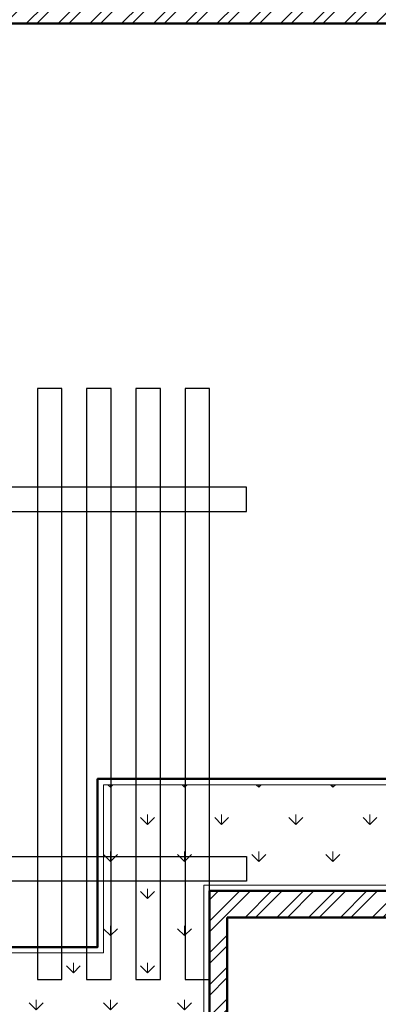
# Model space of a CAD drawing. Units: inches. Extents: x 261 to 2725, y 291 to 1454.
# Tile 28 of 35: x 2144 to 2266, y 467 to 801. Entities that reach past the tile are written whole.
import ezdxf

# ---------------------------------------------------------------- set-up
doc = ezdxf.new("R2010")
doc.units = ezdxf.units.IN
for name, color, linetype, lineweight in [('A-ANNO-DIMS', 136, 'Continuous', 18), ('A-PLNT', 3, 'Continuous', 18), ('A-PLNT-PATT', 3, 'Continuous', 13), ('A-ROOF-PRGL', 25, 'Continuous', 25), ('A-WALL', 222, 'Continuous', 50), ('A-WALL-PATT', 243, 'Continuous', 13)]:
    doc.layers.add(name, color=color, linetype=linetype, lineweight=lineweight)
doc.styles.get("Standard").update_dxf_attribs({"font": 'arial.ttf'})
doc.dimstyles.new('ISO-25', dxfattribs={"dimtxt": 12, "dimasz": 6, "dimexe": 1.25, "dimexo": 0.625, "dimtad": 1, "dimdec": 0, "dimlunit": 3, "dimtxsty": 'Standard', "dimblk": 'ARCHTICK', "dimcen": 2.5, "dimadec": 0, "dimazin": 0, "dimtfac": 1, "dimtdec": 0, "dimtmove": 0, "dimatfit": 3, "dimfxl": 1, "dimfxlon": 1, "dimarcsym": 0})

# ---------------------------------------------------------------- blocks, each defined once
blk = doc.blocks.new('_ArchTick')
at = {"color": 0, "linetype": 'ByBlock', "const_width": 0.15}
blk.add_lwpolyline([(-0.5, -0.5), (0.5, 0.5)], dxfattribs=at)
blk = doc.blocks.new('*D82')
at = {"layer": 'A-ANNO-DIMS', "color": 0, "lineweight": -2, "ltscale": 0.07, "transparency": 16777216}
for p, q in [((2600.96, 679.47), (2603.21, 679.47)), ((2601.96, 517.47), (2601.96, 679.47)), ((2600.96, 517.47), (2603.21, 517.47))]:
    blk.add_line(p, q, dxfattribs=at)
at = {"layer": 'Defpoints', "color": 0, "ltscale": 0.07, "transparency": 16777216}
for p in [(946.45, 679.47), (2601.96, 679.47), (946.45, 517.47)]:
    blk.add_point(p, dxfattribs=at)
at = {"layer": 'A-ANNO-DIMS', "color": 0, "lineweight": -2, "ltscale": 0.07, "transparency": 16777216, "xscale": 6, "yscale": 6, "zscale": 6}
for p, rotation in [((2601.96, 679.47), 90), ((2601.96, 517.47), 270)]:
    blk.add_blockref('_ArchTick', p, dxfattribs=dict(at, rotation=rotation))
at = {"layer": 'A-ANNO-DIMS', "color": 0, "ltscale": 0.07, "transparency": 16777216, "insert": (2595.2, 598.47), "char_height": 12, "attachment_point": 5, "rotation": 90}
blk.add_mtext('13\'-6"', dxfattribs=at)
blk = doc.blocks.new('*D83')
at = {"layer": 'A-ANNO-DIMS', "color": 0, "lineweight": -2, "ltscale": 0.07, "transparency": 16777216}
for p, q in [((2600.96, 799.47), (2603.21, 799.47)), ((2601.96, 679.47), (2601.96, 799.47)), ((2600.96, 679.47), (2603.21, 679.47))]:
    blk.add_line(p, q, dxfattribs=at)
at = {"layer": 'Defpoints', "color": 0, "ltscale": 0.07, "transparency": 16777216}
for p in [(946.45, 799.47), (2601.96, 799.47), (946.45, 679.47)]:
    blk.add_point(p, dxfattribs=at)
at = {"layer": 'A-ANNO-DIMS', "color": 0, "lineweight": -2, "ltscale": 0.07, "transparency": 16777216, "xscale": 6, "yscale": 6, "zscale": 6}
for p, rotation in [((2601.96, 799.47), 90), ((2601.96, 679.47), 270)]:
    blk.add_blockref('_ArchTick', p, dxfattribs=dict(at, rotation=rotation))
at = {"layer": 'A-ANNO-DIMS', "color": 0, "ltscale": 0.07, "transparency": 16777216, "insert": (2595.21, 739.47), "char_height": 12, "attachment_point": 5, "rotation": 90}
blk.add_mtext('10\'-0"', dxfattribs=at)
blk = doc.blocks.new('*D84')
at = {"layer": 'A-ANNO-DIMS', "color": 0, "lineweight": -2, "ltscale": 0.07, "transparency": 16777216}
for p, q in [((2600.96, 1024.47), (2603.21, 1024.47)), ((2601.96, 799.47), (2601.96, 1024.47)), ((2600.96, 799.47), (2603.21, 799.47))]:
    blk.add_line(p, q, dxfattribs=at)
at = {"layer": 'Defpoints', "color": 0, "ltscale": 0.07, "transparency": 16777216}
for p in [(946.45, 1024.47), (2601.96, 1024.47), (946.45, 799.47)]:
    blk.add_point(p, dxfattribs=at)
at = {"layer": 'A-ANNO-DIMS', "color": 0, "lineweight": -2, "ltscale": 0.07, "transparency": 16777216, "xscale": 6, "yscale": 6, "zscale": 6}
for p, rotation in [((2601.96, 1024.47), 90), ((2601.96, 799.47), 270)]:
    blk.add_blockref('_ArchTick', p, dxfattribs=dict(at, rotation=rotation))
at = {"layer": 'A-ANNO-DIMS', "color": 0, "ltscale": 0.07, "transparency": 16777216, "insert": (2595.21, 911.97), "char_height": 12, "attachment_point": 5, "rotation": 90}
blk.add_mtext('18\'-9"', dxfattribs=at)
blk = doc.blocks.new('*D89')
at = {"layer": 'A-ANNO-DIMS', "color": 0, "lineweight": -2, "ltscale": 0.07, "transparency": 16777216}
for p, q in [((2600.96, 508.47), (2603.21, 508.47)), ((2601.96, 412.47), (2601.96, 508.47)), ((2600.96, 412.47), (2603.21, 412.47))]:
    blk.add_line(p, q, dxfattribs=at)
at = {"layer": 'Defpoints', "color": 0, "ltscale": 0.07, "transparency": 16777216}
for p in [(955.45, 508.47), (2601.96, 508.47), (994.45, 412.47)]:
    blk.add_point(p, dxfattribs=at)
at = {"layer": 'A-ANNO-DIMS', "color": 0, "lineweight": -2, "ltscale": 0.07, "transparency": 16777216, "xscale": 6, "yscale": 6, "zscale": 6}
for p, rotation in [((2601.96, 508.47), 90), ((2601.96, 412.47), 270)]:
    blk.add_blockref('_ArchTick', p, dxfattribs=dict(at, rotation=rotation))
at = {"layer": 'A-ANNO-DIMS', "color": 0, "ltscale": 0.07, "transparency": 16777216, "insert": (2595.21, 460.47), "char_height": 12, "attachment_point": 5, "rotation": 90}
blk.add_mtext('8\'-0"', dxfattribs=at)
blk = doc.blocks.new('*D111')
at = {"layer": 'A-ANNO-DIMS', "color": 0, "lineweight": -2, "ltscale": 0.07, "transparency": 16777216}
for p, q in [((2600.96, 550.47), (2603.21, 550.47)), ((2601.96, 448.47), (2601.96, 550.47)), ((2600.96, 448.47), (2603.21, 448.47))]:
    blk.add_line(p, q, dxfattribs=at)
at = {"layer": 'Defpoints', "color": 0, "ltscale": 0.07, "transparency": 16777216}
for p in [(1720.08, 550.47), (2601.96, 550.47), (1720.08, 448.47)]:
    blk.add_point(p, dxfattribs=at)
at = {"layer": 'A-ANNO-DIMS', "color": 0, "lineweight": -2, "ltscale": 0.07, "transparency": 16777216, "xscale": 6, "yscale": 6, "zscale": 6}
for p, rotation in [((2601.96, 550.47), 90), ((2601.96, 448.47), 270)]:
    blk.add_blockref('_ArchTick', p, dxfattribs=dict(at, rotation=rotation))
at = {"layer": 'A-ANNO-DIMS', "color": 0, "ltscale": 0.07, "transparency": 16777216, "insert": (2595.21, 499.47), "char_height": 12, "attachment_point": 5, "rotation": 90}
blk.add_mtext('8\'-6"', dxfattribs=at)
blk = doc.blocks.new('*D112')
at = {"layer": 'A-ANNO-DIMS', "color": 0, "lineweight": -2, "ltscale": 0.07, "transparency": 16777216}
for p, q in [((2600.96, 679.47), (2603.21, 679.47)), ((2601.96, 550.47), (2601.96, 679.47)), ((2600.96, 550.47), (2603.21, 550.47))]:
    blk.add_line(p, q, dxfattribs=at)
at = {"layer": 'Defpoints', "color": 0, "ltscale": 0.07, "transparency": 16777216}
for p in [(1720.08, 679.47), (2601.96, 679.47), (1720.08, 550.47)]:
    blk.add_point(p, dxfattribs=at)
at = {"layer": 'A-ANNO-DIMS', "color": 0, "lineweight": -2, "ltscale": 0.07, "transparency": 16777216, "xscale": 6, "yscale": 6, "zscale": 6}
for p, rotation in [((2601.96, 679.47), 90), ((2601.96, 550.47), 270)]:
    blk.add_blockref('_ArchTick', p, dxfattribs=dict(at, rotation=rotation))
at = {"layer": 'A-ANNO-DIMS', "color": 0, "ltscale": 0.07, "transparency": 16777216, "insert": (2595.21, 614.97), "char_height": 12, "attachment_point": 5, "rotation": 90}
blk.add_mtext('10\'-9"', dxfattribs=at)
blk = doc.blocks.new('*D113')
at = {"layer": 'A-ANNO-DIMS', "color": 0, "lineweight": -2, "ltscale": 0.07, "transparency": 16777216}
for p, q in [((2600.96, 799.47), (2603.21, 799.47)), ((2601.96, 679.47), (2601.96, 799.47)), ((2600.96, 679.47), (2603.21, 679.47))]:
    blk.add_line(p, q, dxfattribs=at)
at = {"layer": 'Defpoints', "color": 0, "ltscale": 0.07, "transparency": 16777216}
for p in [(1720.08, 799.47), (2601.96, 799.47), (1720.08, 679.47)]:
    blk.add_point(p, dxfattribs=at)
at = {"layer": 'A-ANNO-DIMS', "color": 0, "lineweight": -2, "ltscale": 0.07, "transparency": 16777216, "xscale": 6, "yscale": 6, "zscale": 6}
for p, rotation in [((2601.96, 799.47), 90), ((2601.96, 679.47), 270)]:
    blk.add_blockref('_ArchTick', p, dxfattribs=dict(at, rotation=rotation))
at = {"layer": 'A-ANNO-DIMS', "color": 0, "ltscale": 0.07, "transparency": 16777216, "insert": (2595.21, 739.47), "char_height": 12, "attachment_point": 5, "rotation": 90}
blk.add_mtext('10\'-0"', dxfattribs=at)
blk = doc.blocks.new('*D114')
at = {"layer": 'A-ANNO-DIMS', "color": 0, "lineweight": -2, "ltscale": 0.07, "transparency": 16777216}
for p, q in [((2600.96, 964.47), (2603.21, 964.47)), ((2601.96, 799.47), (2601.96, 964.47)), ((2600.96, 799.47), (2603.21, 799.47))]:
    blk.add_line(p, q, dxfattribs=at)
at = {"layer": 'Defpoints', "color": 0, "ltscale": 0.07, "transparency": 16777216}
for p in [(1720.08, 964.47), (2601.96, 964.47), (1720.08, 799.47)]:
    blk.add_point(p, dxfattribs=at)
at = {"layer": 'A-ANNO-DIMS', "color": 0, "lineweight": -2, "ltscale": 0.07, "transparency": 16777216, "xscale": 6, "yscale": 6, "zscale": 6}
for p, rotation in [((2601.96, 964.47), 90), ((2601.96, 799.47), 270)]:
    blk.add_blockref('_ArchTick', p, dxfattribs=dict(at, rotation=rotation))
at = {"layer": 'A-ANNO-DIMS', "color": 0, "ltscale": 0.07, "transparency": 16777216, "insert": (2595.2, 881.97), "char_height": 12, "attachment_point": 5, "rotation": 90}
blk.add_mtext('13\'-9"', dxfattribs=at)
blk = doc.blocks.new('*D125')
at = {"layer": 'A-ANNO-DIMS', "color": 0, "lineweight": -2, "ltscale": 0.07, "transparency": 16777216}
for p, q in [((2600.96, 496.47), (2603.21, 496.47)), ((2601.96, 439.47), (2601.96, 496.47)), ((2600.96, 439.47), (2603.21, 439.47))]:
    blk.add_line(p, q, dxfattribs=at)
at = {"layer": 'Defpoints', "color": 0, "ltscale": 0.07, "transparency": 16777216}
for p in [(2214.67, 496.47), (2601.96, 496.47), (2214.67, 439.47)]:
    blk.add_point(p, dxfattribs=at)
at = {"layer": 'A-ANNO-DIMS', "color": 0, "lineweight": -2, "ltscale": 0.07, "transparency": 16777216, "xscale": 6, "yscale": 6, "zscale": 6}
for p, rotation in [((2601.96, 496.47), 90), ((2601.96, 439.47), 270)]:
    blk.add_blockref('_ArchTick', p, dxfattribs=dict(at, rotation=rotation))
at = {"layer": 'A-ANNO-DIMS', "color": 0, "ltscale": 0.07, "transparency": 16777216, "insert": (2595.21, 467.97), "char_height": 12, "attachment_point": 5, "rotation": 90}
blk.add_mtext('4\'-9"', dxfattribs=at)
blk = doc.blocks.new('*D135')
at = {"layer": 'A-ANNO-DIMS', "color": 0, "lineweight": -2, "ltscale": 0.07, "transparency": 16777216}
for p, q in [((2004.19, 1437.76), (2004.19, 1440.01)), ((2004.19, 1438.76), (2221.19, 1438.76)), ((2221.19, 1437.76), (2221.19, 1440.01))]:
    blk.add_line(p, q, dxfattribs=at)
at = {"layer": 'Defpoints', "color": 0, "ltscale": 0.07, "transparency": 16777216}
for p in [(2221.19, 1438.76), (2004.19, 642.39), (2221.19, 642.39)]:
    blk.add_point(p, dxfattribs=at)
at = {"layer": 'A-ANNO-DIMS', "color": 0, "lineweight": -2, "ltscale": 0.07, "transparency": 16777216, "xscale": 6, "yscale": 6, "zscale": 6, "rotation": 180}
blk.add_blockref('_ArchTick', (2004.19, 1438.76), dxfattribs=at)
at = {"layer": 'A-ANNO-DIMS', "color": 0, "lineweight": -2, "ltscale": 0.07, "transparency": 16777216, "xscale": 6, "yscale": 6, "zscale": 6}
blk.add_blockref('_ArchTick', (2221.19, 1438.76), dxfattribs=at)
at = {"layer": 'A-ANNO-DIMS', "color": 0, "ltscale": 0.07, "transparency": 16777216, "insert": (2112.69, 1445.51), "char_height": 12, "attachment_point": 5}
blk.add_mtext('18\'-1"', dxfattribs=at)
blk = doc.blocks.new('*D136')
at = {"layer": 'A-ANNO-DIMS', "color": 0, "lineweight": -2, "ltscale": 0.07, "transparency": 16777216}
for p, q in [((2600.96, 675.78), (2603.21, 675.78)), ((2601.96, 675.78), (2601.96, 475.47)), ((2600.96, 475.47), (2603.21, 475.47))]:
    blk.add_line(p, q, dxfattribs=at)
at = {"layer": 'Defpoints', "color": 0, "ltscale": 0.07, "transparency": 16777216}
for p in [(2208.67, 675.78), (2208.67, 475.47), (2601.96, 475.47)]:
    blk.add_point(p, dxfattribs=at)
at = {"layer": 'A-ANNO-DIMS', "color": 0, "lineweight": -2, "ltscale": 0.07, "transparency": 16777216, "xscale": 6, "yscale": 6, "zscale": 6}
for p, rotation in [((2601.96, 675.78), 90), ((2601.96, 475.47), 270)]:
    blk.add_blockref('_ArchTick', p, dxfattribs=dict(at, rotation=rotation))
at = {"layer": 'A-ANNO-DIMS', "color": 0, "ltscale": 0.07, "transparency": 16777216, "insert": (2595.13, 575.62), "char_height": 12, "attachment_point": 5, "rotation": 90}
blk.add_mtext('16\'-8 1/2"', dxfattribs=at)
blk = doc.blocks.new('*D137')
at = {"layer": 'A-ANNO-DIMS', "color": 0, "lineweight": -2, "ltscale": 0.07, "transparency": 16777216}
for p, q in [((2600.96, 642.39), (2603.21, 642.39)), ((2601.96, 642.39), (2601.96, 634.05)), ((2600.96, 634.05), (2603.21, 634.05)), ((2601.96, 634.05), (2601.96, 566.94))]:
    blk.add_line(p, q, dxfattribs=at)
at = {"layer": 'Defpoints', "color": 0, "ltscale": 0.07, "transparency": 16777216}
for p in [(2221.19, 642.39), (2221.19, 634.05), (2601.96, 634.05)]:
    blk.add_point(p, dxfattribs=at)
at = {"layer": 'A-ANNO-DIMS', "color": 0, "lineweight": -2, "ltscale": 0.07, "transparency": 16777216, "xscale": 6, "yscale": 6, "zscale": 6}
for p, rotation in [((2601.96, 642.39), 90), ((2601.96, 634.05), 270)]:
    blk.add_blockref('_ArchTick', p, dxfattribs=dict(at, rotation=rotation))
at = {"layer": 'A-ANNO-DIMS', "color": 0, "ltscale": 0.07, "transparency": 16777216, "insert": (2595.13, 597.49), "char_height": 12, "attachment_point": 5, "rotation": 90}
blk.add_mtext('0\'-8 1/2"', dxfattribs=at)
blk = doc.blocks.new('*D138')
at = {"layer": 'A-ANNO-DIMS', "color": 0, "lineweight": -2, "ltscale": 0.07, "transparency": 16777216}
for p, q in [((2600.96, 634.05), (2603.21, 634.05)), ((2601.96, 634.05), (2601.96, 517.2)), ((2600.96, 517.2), (2603.21, 517.2))]:
    blk.add_line(p, q, dxfattribs=at)
at = {"layer": 'Defpoints', "color": 0, "ltscale": 0.07, "transparency": 16777216}
for p in [(2221.19, 634.05), (2221.19, 517.2), (2601.96, 517.2)]:
    blk.add_point(p, dxfattribs=at)
at = {"layer": 'A-ANNO-DIMS', "color": 0, "lineweight": -2, "ltscale": 0.07, "transparency": 16777216, "xscale": 6, "yscale": 6, "zscale": 6}
for p, rotation in [((2601.96, 634.05), 90), ((2601.96, 517.2), 270)]:
    blk.add_blockref('_ArchTick', p, dxfattribs=dict(at, rotation=rotation))
at = {"layer": 'A-ANNO-DIMS', "color": 0, "ltscale": 0.07, "transparency": 16777216, "insert": (2595.21, 575.62), "char_height": 12, "attachment_point": 5, "rotation": 90}
blk.add_mtext('9\'-9"', dxfattribs=at)

msp = doc.modelspace()

# ---------------------------------------------------------------- hatches: boundary and pattern name
at = {"layer": 'A-PLNT-PATT'}
h = msp.add_hatch(dxfattribs=at)
h.set_pattern_fill('GRASS', color=256, scale=0.7)
h.paths.add_polyline_path([(2052.71, 797.47), (2018.71, 797.47), (2018.71, 450.47), (2206.67, 450.47), (2206.67, 507.47), (2482.71, 507.47), (2482.71, 671.47), (2448.71, 671.47), (2448.71, 541.47), (2172.67, 541.47), (2172.67, 484.47), (2052.71, 484.47)])
at = {"layer": 'A-WALL-PATT'}
h = msp.add_hatch(dxfattribs=at)
h.set_pattern_fill('ANSI32', color=256, scale=0.8)
h.paths.add_polyline_path([(478.45, 685.47), (580.45, 685.47), (580.45, 691.47), (577.45, 691.47), (577.45, 694.47), (571.45, 694.47), (571.45, 691.47), (478.45, 691.47), (478.45, 721.47), (469.45, 721.47), (469.45, 508.47), (538.45, 508.47), (538.45, 517.47), (478.45, 517.47)])
h.paths.add_polyline_path([(694.45, 517.47), (676.45, 517.47), (676.45, 646.47), (670.45, 646.47), (670.45, 517.47), (610.45, 517.47), (610.45, 508.47), (694.45, 508.47)])
h.paths.add_polyline_path([(676.45, 784.47), (478.45, 784.47), (478.45, 844.47), (469.45, 844.47), (469.45, 745.47), (478.45, 745.47), (478.45, 775.47), (571.45, 775.47), (571.45, 724.47), (577.45, 724.47), (577.45, 775.47), (670.45, 775.47), (670.45, 691.47), (610.45, 691.47), (610.45, 685.47), (670.45, 685.47), (670.45, 682.47), (676.45, 682.47)])
h.paths.add_polyline_path([(955.45, 880.47), (946.45, 880.47), (946.45, 808.47), (778.45, 808.47), (778.45, 799.47), (946.45, 799.47), (946.45, 517.47), (898.45, 517.47), (898.45, 508.47), (955.45, 508.47)])
h.paths.add_polyline_path([(778.45, 598.47), (772.45, 598.47), (772.45, 517.47), (754.45, 517.47), (754.45, 508.47), (826.45, 508.47), (826.45, 517.47), (778.45, 517.47)])
h.paths.add_polyline_path([(955.45, 1090.47), (946.45, 1090.47), (946.45, 1030.47), (817.45, 1030.47), (817.45, 1024.47), (946.45, 1024.47), (946.45, 952.47), (955.45, 952.47)])
h.paths.add_polyline_path([(955.45, 1231.47), (730.45, 1231.47), (730.45, 1222.47), (772.45, 1222.47), (772.45, 1096.47), (766.45, 1096.47), (766.45, 1090.47), (772.45, 1090.47), (772.45, 1006.47), (712.45, 1006.47), (712.45, 1000.47), (778.45, 1000.47), (778.45, 1024.47), (781.45, 1024.47), (781.45, 1030.47), (778.45, 1030.47), (778.45, 1222.47), (946.45, 1222.47), (946.45, 1162.47), (955.45, 1162.47)])
h.paths.add_polyline_path([(694.45, 1231.47), (619.45, 1231.47), (619.45, 1222.47), (646.45, 1222.47), (646.45, 1039.47), (652.45, 1039.47), (652.45, 1090.47), (736.45, 1090.47), (736.45, 1096.47), (652.45, 1096.47), (652.45, 1222.47), (694.45, 1222.47)])
h.paths.add_polyline_path([(571.45, 1231.47), (469.45, 1231.47), (469.45, 1099.47), (478.45, 1099.47), (478.45, 1144.47), (544.45, 1144.47), (544.45, 1153.47), (538.45, 1153.47), (538.45, 1150.47), (478.45, 1150.47), (478.45, 1222.47), (538.45, 1222.47), (538.45, 1183.47), (544.45, 1183.47), (544.45, 1222.47), (571.45, 1222.47)])
h.paths.add_polyline_path([(538.45, 1006.47), (478.45, 1006.47), (478.45, 1051.47), (469.45, 1051.47), (469.45, 940.47), (478.45, 940.47), (478.45, 1000.47), (538.45, 1000.47)])
h.paths.add_polyline_path([(652.45, 1006.47), (652.45, 1009.47), (646.45, 1009.47), (646.45, 1006.47), (586.45, 1006.47), (586.45, 1000.47), (652.45, 1000.47)])
h.paths.add_polyline_path([(1288.08, 973.47), (1243.08, 973.47), (1243.08, 920.97), (1252.08, 920.97), (1252.08, 964.47), (1288.08, 964.47)], flags=17)
h.paths.add_polyline_path([(1402.08, 805.47), (1252.08, 805.47), (1252.08, 848.97), (1243.08, 848.97), (1243.08, 757.47), (1252.08, 757.47), (1252.08, 799.47), (1294.08, 799.47), (1372.08, 799.47), (1372.08, 779.47), (1372.08, 715.47), (1378.08, 715.47), (1378.08, 799.47), (1402.08, 799.47)])
h.paths.add_polyline_path([(1252.08, 721.47), (1243.08, 721.47), (1243.08, 439.47), (1729.08, 439.47), (1729.08, 709.47), (1720.08, 709.47), (1720.08, 679.47), (1582.08, 679.47), (1582.08, 670.47), (1588.08, 670.47), (1588.08, 673.47), (1720.08, 673.47), (1720.08, 559.47), (1690.08, 559.47), (1690.08, 550.47), (1720.08, 550.47), (1720.08, 448.47), (1252.08, 448.47), (1252.08, 496.47), (1312.08, 496.47), (1312.08, 505.47), (1252.08, 505.47), (1252.08, 673.47), (1405.08, 673.47), (1405.08, 679.47), (1378.08, 679.47), (1378.08, 685.47), (1372.08, 685.47), (1372.08, 679.47), (1252.08, 679.47)])
h.paths.add_polyline_path([(1450.08, 550.47), (1480.08, 550.47), (1480.08, 559.47), (1450.08, 559.47), (1450.08, 679.47), (1441.08, 679.47), (1441.08, 673.47), (1444.08, 673.47), (1444.08, 505.47), (1384.08, 505.47), (1384.08, 496.47), (1450.08, 496.47)], flags=17)
h.paths.add_polyline_path([(1618.08, 559.47), (1588.08, 559.47), (1588.08, 634.47), (1582.08, 634.47), (1582.08, 559.47), (1552.08, 559.47), (1552.08, 550.47), (1618.08, 550.47)], flags=17)
h.paths.add_polyline_path([(1564.08, 964.47), (1630.08, 964.47), (1630.08, 973.47), (1477.08, 973.47), (1477.08, 964.47), (1558.08, 964.47), (1558.08, 926.22), (1558.08, 887.97), (1486.08, 887.97), (1486.08, 881.97), (1558.08, 881.97), (1558.08, 805.47), (1450.08, 805.47), (1450.08, 845.97), (1444.08, 845.97), (1444.08, 805.47), (1438.08, 805.47), (1438.08, 799.47), (1564.08, 799.47)], flags=17)
h.paths.add_polyline_path([(1453.08, 973.47), (1408.08, 973.47), (1408.08, 964.47), (1444.08, 964.47), (1444.08, 881.97), (1450.08, 881.97), (1456.08, 881.97), (1456.08, 887.97), (1450.08, 887.97), (1450.08, 964.47), (1453.08, 964.47)], flags=17)
h.paths.add_polyline_path([(1729.08, 1231.47), (1243.08, 1231.47), (1243.08, 1167.47), (1252.08, 1167.47), (1252.08, 1222.47), (1441.08, 1222.47), (1441.08, 1045.47), (1648.08, 1045.47), (1648.08, 1051.47), (1450.08, 1051.47), (1450.08, 1074.47), (1450.08, 1222.47), (1472.08, 1222.47), (1720.08, 1222.47), (1720.08, 1051.47), (1708.08, 1051.47), (1708.08, 1045.47), (1720.08, 1045.47), (1720.08, 973.47), (1702.08, 973.47), (1702.08, 964.47), (1720.08, 964.47), (1720.08, 769.47), (1729.08, 769.47)])
h.paths.add_polyline_path([(2493.71, 1054.85), (2007.71, 1054.85), (2007.71, 439.47), (2214.67, 439.47), (2214.67, 496.47), (2493.71, 496.47)])
h.paths.add_polyline_path([(2016.71, 1045.85), (2304.71, 1045.85), (2304.71, 841.47), (2310.71, 841.47), (2310.71, 1045.85), (2484.71, 1045.85), (2484.71, 805.47), (2310.71, 805.47), (2310.71, 811.47), (2304.71, 811.47), (2304.71, 799.47), (2484.71, 799.47), (2484.71, 679.47), (2304.71, 679.47), (2304.71, 673.47), (2484.71, 673.47), (2484.71, 505.47), (2208.67, 505.47), (2208.67, 448.47), (2016.71, 448.47), (2016.71, 799.47), (2304.71, 799.47), (2304.71, 805.47), (2016.71, 805.47)], flags=16)

# ---------------------------------------------------------------- linework, layer by layer
at = {"layer": 'A-PLNT'}
for points in [[(2018.71, 797.47), (2018.71, 450.47), (2206.67, 450.47), (2206.67, 507.47), (2482.71, 507.47), (2482.71, 671.47)], [(2052.71, 797.47), (2052.71, 484.47), (2172.67, 484.47), (2172.67, 541.47), (2448.71, 541.47), (2448.71, 671.47)]]:
    msp.add_lwpolyline(points, dxfattribs=at)
at = {"layer": 'A-ROOF-PRGL'}
for points in [[(2150.25, 475.47), (2158.6, 475.47), (2158.6, 675.78), (2150.25, 675.78)], [(2166.94, 475.47), (2175.29, 475.47), (2175.29, 675.78), (2166.94, 675.78)], [(2183.63, 475.47), (2191.98, 475.47), (2191.98, 675.78), (2183.63, 675.78)], [(2200.33, 475.47), (2208.67, 475.47), (2208.67, 675.78), (2200.33, 675.78)], [(2004.19, 634.05), (2221.19, 634.05), (2221.19, 642.39), (2004.19, 642.39)], [(2004.19, 517.2), (2221.19, 517.2), (2221.19, 508.85), (2004.19, 508.85)]]:
    msp.add_lwpolyline(points, close=True, dxfattribs=at)
at = {"layer": 'A-WALL'}
for p, q in [((2016.71, 799.47), (2484.71, 799.47)), ((2214.67, 496.47), (2214.67, 439.47)), ((2214.67, 496.47), (2493.71, 496.47))]:
    msp.add_line(p, q, dxfattribs=at)
for points in [[(2016.71, 799.47), (2016.71, 448.47), (2208.67, 448.47), (2208.67, 505.47), (2484.71, 505.47), (2484.71, 673.47)], [(2054.71, 799.47), (2054.71, 486.47), (2170.67, 486.47), (2170.67, 543.47), (2446.71, 543.47), (2446.71, 673.47)]]:
    msp.add_lwpolyline(points, dxfattribs=at)

# ---------------------------------------------------------------- dimensions: what is measured, and where the dimension line sits
at = {"layer": 'A-ANNO-DIMS', "ltscale": 0.07}
dim = msp.add_linear_dim(base=(2221.19, 1438.76), p1=(2004.19, 642.39), p2=(2221.19, 642.39), dimstyle='ISO-25', override={"dimdec": 1, "dimlfac": 1, "dimrnd": 0, "dimzin": 1, "dimdsep": 46, "dimlunit": 4, "dimfrac": 2}, dxfattribs=at)
dim.commit()
dim.dimension.update_dxf_attribs({"geometry": '*D135', "text_midpoint": (2112.69, 1445.51)})
for base, p1, p2, picture, middle in [((2601.96, 1024.47), (946.45, 799.47), (946.45, 1024.47), '*D84', (2595.21, 911.97)), ((2601.96, 964.47), (1720.08, 799.47), (1720.08, 964.47), '*D114', (2595.2, 881.97)), ((2601.96, 799.47), (946.45, 679.47), (946.45, 799.47), '*D83', (2595.21, 739.47)), ((2601.96, 799.47), (1720.08, 679.47), (1720.08, 799.47), '*D113', (2595.21, 739.47)), ((2601.96, 679.47), (946.45, 517.47), (946.45, 679.47), '*D82', (2595.2, 598.47)), ((2601.96, 679.47), (1720.08, 550.47), (1720.08, 679.47), '*D112', (2595.21, 614.97)), ((2601.96, 475.47), (2208.67, 675.78), (2208.67, 475.47), '*D136', (2595.13, 575.62)), ((2601.96, 634.05), (2221.19, 642.39), (2221.19, 634.05), '*D137', (2595.13, 597.49)), ((2601.9578, 517.1998), (2221.1928, 634.0483), (2221.1928, 517.1998), '*D138', (2595.2059, 575.6241)), ((2601.96, 550.47), (1720.08, 448.47), (1720.08, 550.47), '*D111', (2595.21, 499.47)), ((2601.96, 508.47), (994.45, 412.47), (955.45, 508.47), '*D89', (2595.21, 460.47)), ((2601.96, 496.47), (2214.67, 439.47), (2214.67, 496.47), '*D125', (2595.21, 467.97))]:
    dim = msp.add_linear_dim(base=base, p1=p1, p2=p2, angle=90, dimstyle='ISO-25', override={"dimdec": 1, "dimlfac": 1, "dimrnd": 0, "dimzin": 1, "dimdsep": 46, "dimlunit": 4, "dimfrac": 2}, dxfattribs=at)
    dim.commit()
    dim.dimension.update_dxf_attribs({"geometry": picture, "text_midpoint": middle})

doc.saveas('drawing.dxf')
